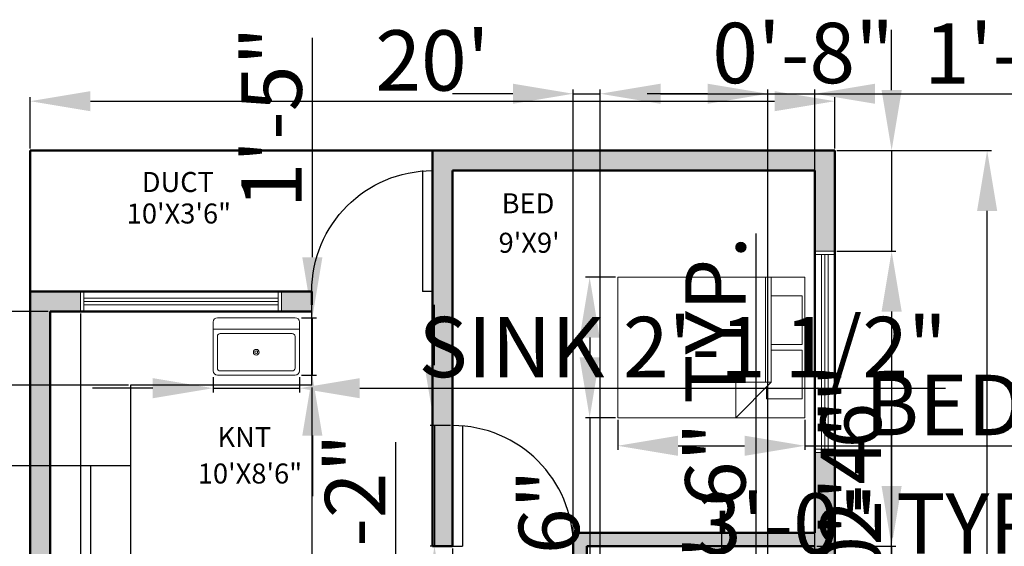
# Model space of a CAD drawing. Units: inches. Extents: x -261 to 409, y 193 to 762.
# Tile 5 of 6: x -35 to 259, y 605 to 762. Entities that reach past the tile are written whole.
import ezdxf

# ---------------------------------------------------------------- set-up
doc = ezdxf.new("R2010")
doc.units = ezdxf.units.IN
for name, color, linetype, lineweight in [('A-ANNO-DIMS', 2, 'Continuous', 18), ('A-AREA-IDEN', 7, 'Continuous', 25), ('A-DOOR', 3, 'Continuous', 25), ('A-FLOR-CASE', 9, 'Continuous', 25), ('A-FLOR-FIXT', 9, 'Continuous', 18), ('A-FURN', 8, 'Continuous', 18), ('A-GLAZ', 4, 'Continuous', 18), ('A-WALL', 7, 'Continuous', 50), ('A-WALL-PATT', 8, 'Continuous', 13)]:
    doc.layers.add(name, color=color, linetype=linetype, lineweight=lineweight)
doc.styles.get("Standard").update_dxf_attribs({"font": 'arial.ttf'})
doc.dimstyles.new('ISO-25', dxfattribs={"dimtxt": 18, "dimasz": 18, "dimexe": 1.25, "dimexo": 0.625, "dimtad": 1, "dimdec": 1, "dimlunit": 3, "dimtxsty": 'Standard', "dimcen": 2.5, "dimadec": 0, "dimazin": 0, "dimtfac": 1, "dimtdec": 1, "dimtmove": 0, "dimatfit": 3, "dimfxl": 1, "dimarcsym": 0})

# ---------------------------------------------------------------- blocks, each defined once
blk = doc.blocks.new('Bed - Queen')
for p, q in [((0, -80.00003), (0, 0)), ((0, 0), (59.99999, 0)), ((59.99999, 0), (59.99999, -80.00003)), ((7.99999, -1.2), (28.79998, -1.2)), ((7.99999, -14.4), (7.99999, -1.2)), ((28.79998, -1.2), (28.79998, -14.4)), ((31.19999, -1.2), (51.99999, -1.2)), ((31.19999, -14.4), (31.19999, -1.2)), ((51.99999, -1.2), (51.99999, -16.4)), ((0, -14.4), (44.8, -14.4)), ((44.8, -16.8), (0, -16.8)), ((59.99999, -29.6), (44.8, -14.4)), ((44.8, -14.4), (44.8, -29.6)), ((51.99999, -16.4), (46.79936, -16.4)), ((44.8, -29.6), (59.99999, -29.6)), ((59.99999, -80.00003), (0, -80.00003))]:
    blk.add_line(p, q)
blk = doc.blocks.new('Sink-single - 30 in top')
blk.add_line((-15, -3.999996), (15, -3.999996))
for points in [[(-13.5, 0), (13.5, 0)], [(-15, -18.499996), (-15, -1.5)], [(15, -1.5), (15, -18.499996)], [(-13.5, -17.499996), (-13.5, -6.499996)], [(-12.5, -5.499996), (12.5, -5.499996)], [(13.5, -6.499996), (13.5, -17.499996)], [(13.5, -19.999996), (-13.5, -19.999996)], [(12.5, -18.499996), (-12.5, -18.499996)]]:
    blk.add_lwpolyline(points)
for radius in [1, 0.5]:
    blk.add_circle((0, -11.999996), radius)
for centre, radius, start, end in [((-13.5, -1.5), 1.5, 90, 180), ((13.5, -1.5), 1.5, 0, 90), ((-12.5, -6.499996), 1, 90, 180), ((12.5, -6.499996), 1, 0, 90), ((-13.5, -18.499996), 1.5, 180, 270), ((-12.5, -17.499996), 1, 180, 270), ((12.5, -17.499996), 1, 270, 0), ((13.5, -18.499996), 1.5, 270, 0)]:
    blk.add_arc(centre, radius, start, end)
blk = doc.blocks.new('*D5')
at = {"layer": 'A-ANNO-DIMS', "color": 0, "lineweight": -2, "transparency": 16777216}
for p, q in [((-31.7, 723.89), (-31.7, 739.21)), ((-13.7, 737.96), (190.3, 737.96)), ((208.3, 723.89), (208.3, 739.21))]:
    blk.add_line(p, q, dxfattribs=at)
at = {"layer": 'A-ANNO-DIMS', "color": 0, "transparency": 16777216}
for points in [[(-13.7, 740.96), (-13.7, 734.96), (-31.7, 737.96)], [(190.3, 740.96), (190.3, 734.96), (208.3, 737.96)]]:
    blk.add_solid(points, dxfattribs=at)
at = {"layer": 'Defpoints', "color": 0, "transparency": 16777216}
for p in [(208.3, 737.96), (-31.7, 723.26), (208.3, 723.26)]:
    blk.add_point(p, dxfattribs=at)
at = {"layer": 'A-ANNO-DIMS', "color": 0, "transparency": 16777216, "insert": (88.3, 747.77), "char_height": 18, "attachment_point": 5}
blk.add_mtext("20'", dxfattribs=at)
blk = doc.blocks.new('*D6')
at = {"layer": 'A-ANNO-DIMS', "color": 0, "lineweight": -2, "transparency": 16777216}
for p, q in [((208.93, 723.26), (254.96, 723.26)), ((253.71, 441.26), (253.71, 705.26)), ((208.93, 423.26), (254.96, 423.26))]:
    blk.add_line(p, q, dxfattribs=at)
at = {"layer": 'A-ANNO-DIMS', "color": 0, "transparency": 16777216}
for points in [[(250.71, 705.26), (256.71, 705.26), (253.71, 723.26)], [(250.71, 441.26), (256.71, 441.26), (253.71, 423.26)]]:
    blk.add_solid(points, dxfattribs=at)
at = {"layer": 'Defpoints', "color": 0, "transparency": 16777216}
for p in [(208.3, 723.26), (253.71, 723.26), (208.3, 423.26)]:
    blk.add_point(p, dxfattribs=at)
at = {"layer": 'A-ANNO-DIMS', "color": 0, "transparency": 16777216, "insert": (243.89, 573.26), "char_height": 18, "attachment_point": 5, "rotation": 90}
blk.add_mtext("25'", dxfattribs=at)
blk = doc.blocks.new('DOOR-SWING-36IN')
for p, q in [((0, 3), (36, 3)), ((36, 0), (36, 3)), ((0, 0), (36, 0))]:
    blk.add_line(p, q)
blk.add_arc((36, 0), 36, 90, 180)
blk = doc.blocks.new('WIN-60IN')
for p, q in [((60, 6), (0, 6)), ((0, 6), (0, 0)), ((1, 6), (1, 0)), ((59, 0), (59, 6)), ((60, 0), (60, 6)), ((59, 4), (1, 4)), ((59, 3), (1, 3)), ((0, 0), (60, 0)), ((59, 2), (1, 2))]:
    blk.add_line(p, q)
blk = doc.blocks.new('*D11')
at = {"layer": 'A-ANNO-DIMS', "color": 0, "lineweight": -2, "transparency": 16777216}
for p, q in [((88.9, 659.26), (88.9, 677.26)), ((93.68, 641.26), (87.65, 641.26)), ((88.9, 641.26), (88.9, 605.26)), ((93.68, 605.26), (87.65, 605.26)), ((88.9, 587.26), (88.9, 376.77))]:
    blk.add_line(p, q, dxfattribs=at)
at = {"layer": 'A-ANNO-DIMS', "color": 0, "transparency": 16777216}
for points in [[(85.9, 659.26), (91.9, 659.26), (88.9, 641.26)], [(85.9, 587.26), (91.9, 587.26), (88.9, 605.26)]]:
    blk.add_solid(points, dxfattribs=at)
at = {"layer": 'Defpoints', "color": 0, "transparency": 16777216}
for p in [(94.3, 641.26), (88.9, 605.26), (94.3, 605.26)]:
    blk.add_point(p, dxfattribs=at)
at = {"layer": 'A-ANNO-DIMS', "color": 0, "transparency": 16777216, "insert": (78.96, 473.02), "char_height": 18, "attachment_point": 5, "rotation": 90}
blk.add_mtext('DOOR 3\'-0" TYP.', dxfattribs=at)
blk = doc.blocks.new('*D12')
at = {"layer": 'A-ANNO-DIMS', "color": 0, "lineweight": -2, "transparency": 16777216}
for p, q in [((94.3, 604.64), (94.3, 598.61)), ((130.3, 604.64), (130.3, 598.61)), ((76.3, 599.86), (58.3, 599.86)), ((94.3, 599.86), (130.3, 599.86)), ((148.3, 599.86), (277.26, 599.86))]:
    blk.add_line(p, q, dxfattribs=at)
at = {"layer": 'A-ANNO-DIMS', "color": 0, "transparency": 16777216}
for points in [[(76.3, 602.86), (76.3, 596.86), (94.3, 599.86)], [(148.3, 602.86), (148.3, 596.86), (130.3, 599.86)]]:
    blk.add_solid(points, dxfattribs=at)
at = {"layer": 'Defpoints', "color": 0, "transparency": 16777216}
for p in [(94.3, 605.26), (130.3, 605.26), (130.3, 599.86)]:
    blk.add_point(p, dxfattribs=at)
at = {"layer": 'A-ANNO-DIMS', "color": 0, "transparency": 16777216, "insert": (221.78, 609.69), "char_height": 18, "attachment_point": 5}
blk.add_mtext('3\'-0" TYP.', dxfattribs=at)
blk = doc.blocks.new('*D14')
at = {"layer": 'A-ANNO-DIMS', "color": 0, "lineweight": -2, "transparency": 16777216}
for p, q in [((184.8, 569.26), (184.8, 698.54)), ((180.93, 551.26), (186.05, 551.26)), ((184.8, 521.26), (184.8, 551.26)), ((180.93, 521.26), (186.05, 521.26)), ((184.8, 503.26), (184.8, 485.26))]:
    blk.add_line(p, q, dxfattribs=at)
at = {"layer": 'A-ANNO-DIMS', "color": 0, "transparency": 16777216}
for points in [[(181.8, 569.26), (187.8, 569.26), (184.8, 551.26)], [(181.8, 503.26), (187.8, 503.26), (184.8, 521.26)]]:
    blk.add_solid(points, dxfattribs=at)
at = {"layer": 'Defpoints', "color": 0, "transparency": 16777216}
for p in [(180.3, 551.26), (184.8, 551.26), (180.3, 521.26)]:
    blk.add_point(p, dxfattribs=at)
at = {"layer": 'A-ANNO-DIMS', "color": 0, "transparency": 16777216, "insert": (174.99, 642.9), "char_height": 18, "attachment_point": 5, "rotation": 90}
blk.add_mtext('2\'-6" TYP.', dxfattribs=at)
blk = doc.blocks.new('*D19')
at = {"layer": 'A-ANNO-DIMS', "color": 0, "lineweight": -2, "transparency": 16777216}
for p, q in [((143.56, 642.98), (143.56, 633.98)), ((199.37, 642.98), (199.37, 633.98)), ((161.56, 635.23), (181.37, 635.23)), ((199.37, 635.23), (324.36, 635.23))]:
    blk.add_line(p, q, dxfattribs=at)
at = {"layer": 'A-ANNO-DIMS', "color": 0, "transparency": 16777216}
for points in [[(161.56, 638.23), (161.56, 632.23), (143.56, 635.23)], [(181.37, 638.23), (181.37, 632.23), (199.37, 635.23)]]:
    blk.add_solid(points, dxfattribs=at)
at = {"layer": 'Defpoints', "color": 0, "transparency": 16777216}
for p in [(143.56, 643.61), (199.37, 643.61), (199.37, 635.23)]:
    blk.add_point(p, dxfattribs=at)
at = {"layer": 'A-ANNO-DIMS', "color": 0, "transparency": 16777216, "insert": (270.87, 645.05), "char_height": 18, "attachment_point": 5}
blk.add_mtext('BED 4\'-8"', dxfattribs=at)
blk = doc.blocks.new('*D20')
at = {"layer": 'A-ANNO-DIMS', "color": 0, "lineweight": -2, "transparency": 16777216}
for p, q in [((142.93, 685.47), (133.93, 685.47)), ((135.18, 667.47), (135.18, 661.61)), ((142.93, 643.61), (133.93, 643.61)), ((135.18, 643.61), (135.18, 576.52))]:
    blk.add_line(p, q, dxfattribs=at)
at = {"layer": 'A-ANNO-DIMS', "color": 0, "transparency": 16777216}
for points in [[(132.18, 667.47), (138.18, 667.47), (135.18, 685.47)], [(132.18, 661.61), (138.18, 661.61), (135.18, 643.61)]]:
    blk.add_solid(points, dxfattribs=at)
at = {"layer": 'Defpoints', "color": 0, "transparency": 16777216}
for p in [(143.56, 685.47), (135.18, 643.61), (143.56, 643.61)]:
    blk.add_point(p, dxfattribs=at)
at = {"layer": 'A-ANNO-DIMS', "color": 0, "transparency": 16777216, "insert": (125.36, 601.06), "char_height": 18, "attachment_point": 5, "rotation": 90}
blk.add_mtext('3\'-6"', dxfattribs=at)
blk = doc.blocks.new('*D23')
at = {"layer": 'A-ANNO-DIMS', "color": 0, "lineweight": -2, "transparency": 16777216}
for p, q in [((174.57, 597.13), (174.57, 615.13)), ((176.57, 579.13), (173.32, 579.13)), ((174.57, 579.13), (174.57, 561.62)), ((176.57, 561.62), (173.32, 561.62)), ((174.57, 543.62), (174.57, 384.96))]:
    blk.add_line(p, q, dxfattribs=at)
at = {"layer": 'A-ANNO-DIMS', "color": 0, "transparency": 16777216}
for points in [[(171.57, 597.13), (177.57, 597.13), (174.57, 579.13)], [(171.57, 543.62), (177.57, 543.62), (174.57, 561.62)]]:
    blk.add_solid(points, dxfattribs=at)
at = {"layer": 'Defpoints', "color": 0, "transparency": 16777216}
for p in [(177.2, 579.13), (174.57, 561.62), (177.2, 561.62)]:
    blk.add_point(p, dxfattribs=at)
at = {"layer": 'A-ANNO-DIMS', "color": 0, "transparency": 16777216, "insert": (164.64, 455.29), "char_height": 18, "attachment_point": 5, "rotation": 90}
blk.add_mtext('WC 1\'-5 1/2"', dxfattribs=at)
blk = doc.blocks.new('*D25')
at = {"layer": 'A-ANNO-DIMS', "color": 0, "lineweight": -2, "transparency": 16777216}
for p, q in [((22.88, 655.64), (22.88, 651.15)), ((48.62, 655.64), (48.62, 651.15)), ((4.88, 652.4), (-13.12, 652.4)), ((22.88, 652.4), (48.62, 652.4)), ((66.62, 652.4), (241.26, 652.4))]:
    blk.add_line(p, q, dxfattribs=at)
at = {"layer": 'A-ANNO-DIMS', "color": 0, "transparency": 16777216}
for points in [[(4.88, 655.4), (4.88, 649.4), (22.88, 652.4)], [(66.62, 655.4), (66.62, 649.4), (48.62, 652.4)]]:
    blk.add_solid(points, dxfattribs=at)
at = {"layer": 'Defpoints', "color": 0, "transparency": 16777216}
for p in [(22.88, 656.26), (48.62, 656.26), (48.62, 652.4)]:
    blk.add_point(p, dxfattribs=at)
at = {"layer": 'A-ANNO-DIMS', "color": 0, "transparency": 16777216, "insert": (162.94, 662.33), "char_height": 18, "attachment_point": 5}
blk.add_mtext('SINK 2\'-1 1/2"', dxfattribs=at)
blk = doc.blocks.new('*D26')
at = {"layer": 'A-ANNO-DIMS', "color": 0, "lineweight": -2, "transparency": 16777216}
for p, q in [((52.48, 691.42), (52.48, 756.83)), ((49.25, 673.42), (53.73, 673.42)), ((52.48, 656.26), (52.48, 673.42)), ((49.25, 656.26), (53.73, 656.26)), ((52.48, 638.26), (52.48, 620.26))]:
    blk.add_line(p, q, dxfattribs=at)
at = {"layer": 'A-ANNO-DIMS', "color": 0, "transparency": 16777216}
for points in [[(49.48, 691.42), (55.48, 691.42), (52.48, 673.42)], [(49.48, 638.26), (55.48, 638.26), (52.48, 656.26)]]:
    blk.add_solid(points, dxfattribs=at)
at = {"layer": 'Defpoints', "color": 0, "transparency": 16777216}
for p in [(48.62, 673.42), (52.48, 673.42), (48.62, 656.26)]:
    blk.add_point(p, dxfattribs=at)
at = {"layer": 'A-ANNO-DIMS', "color": 0, "transparency": 16777216, "insert": (42.67, 733.12), "char_height": 18, "attachment_point": 5, "rotation": 90}
blk.add_mtext('1\'-5"', dxfattribs=at)
blk = doc.blocks.new('*D30')
at = {"layer": 'A-ANNO-DIMS', "color": 0, "lineweight": -2, "transparency": 16777216}
for p, q in [((225.22, 741.26), (225.22, 759.26)), ((208.93, 723.26), (226.47, 723.26)), ((225.22, 723.26), (225.22, 693.26)), ((208.93, 693.26), (226.47, 693.26)), ((225.22, 675.26), (225.22, 607.86))]:
    blk.add_line(p, q, dxfattribs=at)
at = {"layer": 'A-ANNO-DIMS', "color": 0, "transparency": 16777216}
for points in [[(222.22, 741.26), (228.22, 741.26), (225.22, 723.26)], [(222.22, 675.26), (228.22, 675.26), (225.22, 693.26)]]:
    blk.add_solid(points, dxfattribs=at)
at = {"layer": 'Defpoints', "color": 0, "transparency": 16777216}
for p in [(208.3, 723.26), (208.3, 693.26), (225.22, 693.26)]:
    blk.add_point(p, dxfattribs=at)
at = {"layer": 'A-ANNO-DIMS', "color": 0, "transparency": 16777216, "insert": (215.4, 632.56), "char_height": 18, "attachment_point": 5, "rotation": 90}
blk.add_mtext('2\'-6"', dxfattribs=at)
blk = doc.blocks.new('*D31')
at = {"layer": 'A-ANNO-DIMS', "color": 0, "lineweight": -2, "transparency": 16777216}
for p, q in [((-25.7, 674.64), (-25.7, 405.1)), ((-16.7, 674.64), (-16.7, 405.1)), ((-43.7, 406.35), (-61.7, 406.35)), ((-25.7, 406.35), (-16.7, 406.35)), ((1.3, 406.35), (68.4, 406.35))]:
    blk.add_line(p, q, dxfattribs=at)
at = {"layer": 'A-ANNO-DIMS', "color": 0, "transparency": 16777216}
for points in [[(-43.7, 409.35), (-43.7, 403.35), (-25.7, 406.35)], [(1.3, 409.35), (1.3, 403.35), (-16.7, 406.35)]]:
    blk.add_solid(points, dxfattribs=at)
at = {"layer": 'Defpoints', "color": 0, "transparency": 16777216}
for p in [(-25.7, 675.26), (-16.7, 675.26), (-16.7, 406.35)]:
    blk.add_point(p, dxfattribs=at)
at = {"layer": 'A-ANNO-DIMS', "color": 0, "transparency": 16777216, "insert": (43.85, 416.17), "char_height": 18, "attachment_point": 5}
blk.add_mtext('0\'-9"', dxfattribs=at)
blk = doc.blocks.new('*D33')
at = {"layer": 'A-ANNO-DIMS', "color": 0, "lineweight": -2, "transparency": 16777216}
for p, q in [((225.22, 623.26), (225.22, 641.26)), ((202.93, 605.26), (226.47, 605.26)), ((225.22, 605.26), (225.22, 589.26)), ((202.93, 589.26), (226.47, 589.26)), ((225.22, 571.26), (225.22, 505.86))]:
    blk.add_line(p, q, dxfattribs=at)
at = {"layer": 'A-ANNO-DIMS', "color": 0, "transparency": 16777216}
for points in [[(222.22, 623.26), (228.22, 623.26), (225.22, 605.26)], [(222.22, 571.26), (228.22, 571.26), (225.22, 589.26)]]:
    blk.add_solid(points, dxfattribs=at)
at = {"layer": 'Defpoints', "color": 0, "transparency": 16777216}
for p in [(202.3, 605.26), (202.3, 589.26), (225.22, 589.26)]:
    blk.add_point(p, dxfattribs=at)
at = {"layer": 'A-ANNO-DIMS', "color": 0, "transparency": 16777216, "insert": (215.55, 529.56), "char_height": 18, "attachment_point": 5, "rotation": 90}
blk.add_mtext('1\'-4"', dxfattribs=at)
blk = doc.blocks.new('*D35')
at = {"layer": 'A-ANNO-DIMS', "color": 0, "lineweight": -2, "transparency": 16777216}
for p, q in [((-48.61, 671.26), (-48.61, 689.26)), ((-2.32, 653.26), (-49.86, 653.26)), ((-48.61, 653.26), (-48.61, 629.26)), ((-2.32, 629.26), (-49.86, 629.26)), ((-48.61, 611.26), (-48.61, 543.86))]:
    blk.add_line(p, q, dxfattribs=at)
at = {"layer": 'A-ANNO-DIMS', "color": 0, "transparency": 16777216}
for points in [[(-51.61, 671.26), (-45.61, 671.26), (-48.61, 653.26)], [(-51.61, 611.26), (-45.61, 611.26), (-48.61, 629.26)]]:
    blk.add_solid(points, dxfattribs=at)
at = {"layer": 'Defpoints', "color": 0, "transparency": 16777216}
for p in [(-1.7, 653.26), (-48.61, 629.26), (-1.7, 629.26)]:
    blk.add_point(p, dxfattribs=at)
at = {"layer": 'A-ANNO-DIMS', "color": 0, "transparency": 16777216, "insert": (-58.42, 568.56), "char_height": 18, "attachment_point": 5, "rotation": 90}
blk.add_mtext('2\'-0"', dxfattribs=at)
blk = doc.blocks.new('*D36')
at = {"layer": 'A-ANNO-DIMS', "color": 0, "lineweight": -2, "transparency": 16777216}
for p, q in [((-25.7, 628.64), (-25.7, 405.1)), ((-1.7, 628.64), (-1.7, 405.1)), ((-43.7, 406.35), (-61.7, 406.35)), ((-25.7, 406.35), (-1.7, 406.35)), ((16.3, 406.35), (83.71, 406.35))]:
    blk.add_line(p, q, dxfattribs=at)
at = {"layer": 'A-ANNO-DIMS', "color": 0, "transparency": 16777216}
for points in [[(-43.7, 409.35), (-43.7, 403.35), (-25.7, 406.35)], [(16.3, 409.35), (16.3, 403.35), (-1.7, 406.35)]]:
    blk.add_solid(points, dxfattribs=at)
at = {"layer": 'Defpoints', "color": 0, "transparency": 16777216}
for p in [(-25.7, 629.26), (-1.7, 629.26), (-1.7, 406.35)]:
    blk.add_point(p, dxfattribs=at)
at = {"layer": 'A-ANNO-DIMS', "color": 0, "transparency": 16777216, "insert": (59.01, 416.17), "char_height": 18, "attachment_point": 5}
blk.add_mtext('2\'-0"', dxfattribs=at)
blk = doc.blocks.new('*D38')
at = {"layer": 'A-ANNO-DIMS', "color": 0, "lineweight": -2, "transparency": 16777216}
for p, q in [((225.22, 579.26), (225.22, 646.36)), ((202.93, 561.26), (226.47, 561.26)), ((225.22, 557.26), (225.22, 561.26)), ((202.93, 557.26), (226.47, 557.26)), ((225.22, 539.26), (225.22, 521.26))]:
    blk.add_line(p, q, dxfattribs=at)
at = {"layer": 'A-ANNO-DIMS', "color": 0, "transparency": 16777216}
for points in [[(222.22, 579.26), (228.22, 579.26), (225.22, 561.26)], [(222.22, 539.26), (228.22, 539.26), (225.22, 557.26)]]:
    blk.add_solid(points, dxfattribs=at)
at = {"layer": 'Defpoints', "color": 0, "transparency": 16777216}
for p in [(202.3, 561.26), (225.22, 561.26), (202.3, 557.26)]:
    blk.add_point(p, dxfattribs=at)
at = {"layer": 'A-ANNO-DIMS', "color": 0, "transparency": 16777216, "insert": (215.4, 621.81), "char_height": 18, "attachment_point": 5, "rotation": 90}
blk.add_mtext('0\'-4"', dxfattribs=at)
blk = doc.blocks.new('*D42')
at = {"layer": 'A-ANNO-DIMS', "color": 0, "lineweight": -2, "transparency": 16777216}
for p, q in [((112.3, 740.18), (94.3, 740.18)), ((130.3, 461.89), (130.3, 741.43)), ((130.3, 740.18), (138.3, 740.18)), ((138.3, 461.89), (138.3, 741.43)), ((156.3, 740.18), (223.4, 740.18))]:
    blk.add_line(p, q, dxfattribs=at)
at = {"layer": 'A-ANNO-DIMS', "color": 0, "transparency": 16777216}
for points in [[(112.3, 743.18), (112.3, 737.18), (130.3, 740.18)], [(156.3, 743.18), (156.3, 737.18), (138.3, 740.18)]]:
    blk.add_solid(points, dxfattribs=at)
at = {"layer": 'Defpoints', "color": 0, "transparency": 16777216}
for p in [(138.3, 740.18), (130.3, 461.26), (138.3, 461.26)]:
    blk.add_point(p, dxfattribs=at)
at = {"layer": 'A-ANNO-DIMS', "color": 0, "transparency": 16777216, "insert": (198.85, 749.99), "char_height": 18, "attachment_point": 5}
blk.add_mtext('0\'-8"', dxfattribs=at)
blk = doc.blocks.new('*D43')
at = {"layer": 'A-ANNO-DIMS', "color": 0, "lineweight": -2, "transparency": 16777216}
for p, q in [((77.39, 569.26), (77.39, 636.35)), ((93.68, 569.26), (76.14, 569.26)), ((77.39, 549.26), (77.39, 551.26)), ((93.68, 531.26), (76.14, 531.26))]:
    blk.add_line(p, q, dxfattribs=at)
at = {"layer": 'A-ANNO-DIMS', "color": 0, "transparency": 16777216}
for points in [[(74.39, 551.26), (80.39, 551.26), (77.39, 569.26)], [(74.39, 549.26), (80.39, 549.26), (77.39, 531.26)]]:
    blk.add_solid(points, dxfattribs=at)
at = {"layer": 'Defpoints', "color": 0, "transparency": 16777216}
for p in [(77.39, 569.26), (94.3, 569.26), (94.3, 531.26)]:
    blk.add_point(p, dxfattribs=at)
at = {"layer": 'A-ANNO-DIMS', "color": 0, "transparency": 16777216, "insert": (67.57, 611.81), "char_height": 18, "attachment_point": 5, "rotation": 90}
blk.add_mtext('3\'-2"', dxfattribs=at)
blk = doc.blocks.new('*D44')
at = {"layer": 'A-ANNO-DIMS', "color": 0, "lineweight": -2, "transparency": 16777216}
for p, q in [((170.32, 740.18), (152.32, 740.18)), ((188.32, 562.25), (188.32, 741.43)), ((188.32, 740.18), (202.3, 740.18)), ((202.3, 561.89), (202.3, 741.43)), ((220.3, 740.18), (285.71, 740.18))]:
    blk.add_line(p, q, dxfattribs=at)
at = {"layer": 'A-ANNO-DIMS', "color": 0, "transparency": 16777216}
for points in [[(170.32, 743.18), (170.32, 737.18), (188.32, 740.18)], [(220.3, 743.18), (220.3, 737.18), (202.3, 740.18)]]:
    blk.add_solid(points, dxfattribs=at)
at = {"layer": 'Defpoints', "color": 0, "transparency": 16777216}
for p in [(202.3, 740.18), (188.32, 561.62), (202.3, 561.26)]:
    blk.add_point(p, dxfattribs=at)
at = {"layer": 'A-ANNO-DIMS', "color": 0, "transparency": 16777216, "insert": (262.01, 749.84), "char_height": 18, "attachment_point": 5}
blk.add_mtext('1\'-2"', dxfattribs=at)
blk = doc.blocks.new('*D45')
at = {"layer": 'A-ANNO-DIMS', "color": 0, "lineweight": -2, "transparency": 16777216}
for p, q in [((-48.61, 693.26), (-48.61, 711.26)), ((-26.32, 675.26), (-49.86, 675.26)), ((-48.61, 675.26), (-48.61, 653.26)), ((-2.32, 653.26), (-49.86, 653.26)), ((-48.61, 635.26), (-48.61, 555.87))]:
    blk.add_line(p, q, dxfattribs=at)
at = {"layer": 'A-ANNO-DIMS', "color": 0, "transparency": 16777216}
for points in [[(-51.61, 693.26), (-45.61, 693.26), (-48.61, 675.26)], [(-51.61, 635.26), (-45.61, 635.26), (-48.61, 653.26)]]:
    blk.add_solid(points, dxfattribs=at)
at = {"layer": 'Defpoints', "color": 0, "transparency": 16777216}
for p in [(-25.7, 675.26), (-48.61, 653.26), (-1.7, 653.26)]:
    blk.add_point(p, dxfattribs=at)
at = {"layer": 'A-ANNO-DIMS', "color": 0, "transparency": 16777216, "insert": (-58.42, 586.57), "char_height": 18, "attachment_point": 5, "rotation": 90}
blk.add_mtext('1\'-10"', dxfattribs=at)
blk = doc.blocks.new('*D46')
at = {"layer": 'A-ANNO-DIMS', "color": 0, "lineweight": -2, "transparency": 16777216}
for p, q in [((-1.7, 652.64), (-1.7, 405.1)), ((52.3, 652.64), (52.3, 405.1)), ((16.3, 406.35), (34.3, 406.35))]:
    blk.add_line(p, q, dxfattribs=at)
at = {"layer": 'A-ANNO-DIMS', "color": 0, "transparency": 16777216}
for points in [[(16.3, 409.35), (16.3, 403.35), (-1.7, 406.35)], [(34.3, 409.35), (34.3, 403.35), (52.3, 406.35)]]:
    blk.add_solid(points, dxfattribs=at)
at = {"layer": 'Defpoints', "color": 0, "transparency": 16777216}
for p in [(-1.7, 653.26), (52.3, 653.26), (52.3, 406.35)]:
    blk.add_point(p, dxfattribs=at)
at = {"layer": 'A-ANNO-DIMS', "color": 0, "transparency": 16777216, "insert": (25.3, 416.17), "char_height": 18, "attachment_point": 5}
blk.add_mtext('4\'-6"', dxfattribs=at)

msp = doc.modelspace()

# ---------------------------------------------------------------- hatches: boundary and pattern name
at = {"layer": 'A-WALL-PATT'}
h = msp.add_hatch(color=256, dxfattribs=at)
h.dxf.hatch_style = 1
h.paths.add_polyline_path([(-25.7, 675.26), (-16.7, 675.26), (-16.7, 681.26), (-31.7, 681.26), (-31.7, 423.26), (-14.2, 423.26), (-14.2, 429.26), (-25.7, 429.26), (-25.7, 569.26), (52.3, 569.26), (88.3, 569.26), (94.3, 569.26), (94.3, 573.26), (52.3, 573.26), (-25.7, 573.26), (-25.7, 575.26)])
h.paths.add_polyline_path([(94.3, 429.26), (58.3, 429.26), (45.8, 429.26), (45.8, 423.26), (94.3, 423.26)])
h.paths.add_polyline_path([(208.3, 533.26), (202.3, 533.26), (202.3, 521.26), (150.3, 521.26), (94.3, 521.26), (94.3, 531.26), (88.3, 531.26), (88.3, 465.26), (94.3, 465.26), (94.3, 517.26), (150.3, 517.26), (202.3, 517.26), (202.3, 429.26), (130.3, 429.26), (130.3, 423.26), (208.3, 423.26)])
h.paths.add_polyline_path([(208.3, 577.26), (202.3, 577.26), (202.3, 561.26), (130.3, 561.26), (130.3, 557.26), (150.3, 557.26), (150.3, 551.26), (154.3, 551.26), (154.3, 557.26), (202.3, 557.26), (202.3, 545.26), (208.3, 545.26)])
h.paths.add_polyline_path([(208.3, 633.26), (202.3, 633.26), (202.3, 609.26), (130.3, 609.26), (130.3, 605.26), (130.3, 591.26), (134.3, 591.26), (134.3, 605.26), (202.3, 605.26), (202.3, 589.26), (208.3, 589.26)])
h.paths.add_polyline_path([(208.3, 723.26), (88.3, 723.26), (88.3, 605.26), (94.3, 605.26), (94.3, 641.26), (94.3, 717.26), (202.3, 717.26), (202.3, 693.26), (208.3, 693.26)])
h.paths.add_polyline_path([(52.3, 681.26), (43.3, 681.26), (43.3, 675.26), (52.3, 675.26), (52.3, 677.26)], flags=17)

# ---------------------------------------------------------------- linework, layer by layer
at = {"layer": 'A-FLOR-CASE'}
for p, q in [((52.3, 653.26), (52.3, 677.26)), ((-1.7, 653.26), (-1.7, 629.26)), ((52.3, 653.26), (-1.7, 653.26)), ((-1.7, 629.26), (-25.7, 629.26)), ((-13.7, 629.26), (-13.7, 579.26))]:
    msp.add_line(p, q, dxfattribs=at)
at = {"layer": 'A-WALL'}
for p, q in [((208.3, 723.26), (-31.7, 723.26)), ((-31.7, 723.26), (-31.7, 423.26)), ((88.3, 723.26), (88.3, 605.26)), ((208.3, 423.26), (208.3, 723.26)), ((94.3, 717.26), (94.3, 605.26)), ((202.3, 717.26), (94.3, 717.26)), ((202.3, 609.26), (202.3, 717.26)), ((52.3, 681.26), (-31.7, 681.26)), ((52.3, 681.26), (52.3, 677.26)), ((-25.7, 675.26), (-25.7, 575.26)), ((52.3, 675.26), (-25.7, 675.26)), ((202.3, 609.26), (130.3, 609.26)), ((130.3, 609.26), (130.3, 605.26)), ((94.3, 605.26), (88.3, 605.26)), ((130.3, 591.26), (130.3, 605.26)), ((202.3, 605.26), (134.3, 605.26)), ((134.3, 591.26), (134.3, 605.26))]:
    msp.add_line(p, q, dxfattribs=at)

# ---------------------------------------------------------------- block references
at = {"layer": 'A-DOOR', "extrusion": (0, 0, -1), "zscale": -1, "rotation": 270}
msp.add_blockref('DOOR-SWING-36IN', (-88.3, 717.26), dxfattribs=at)
at = {"layer": 'A-DOOR', "rotation": 270}
msp.add_blockref('DOOR-SWING-36IN', (94.3, 641.26), dxfattribs=at)
at = {"layer": 'A-FLOR-FIXT', "xscale": 0.8579498762486251, "yscale": 0.8579498762486251, "zscale": 0.8579498762486251}
msp.add_blockref('Sink-single - 30 in top', (35.75, 673.42), dxfattribs=at)
at = {"layer": 'A-FURN', "xscale": 0.6976867227961034, "yscale": 0.6976867227961034, "zscale": 0.6976867227961034, "rotation": 270}
msp.add_blockref('Bed - Queen', (199.37, 685.47), dxfattribs=at)
at = {"layer": 'A-GLAZ'}
for p, rotation in [((202.3, 693.26), 270.0000000000004), ((43.3, 681.26), 180)]:
    msp.add_blockref('WIN-60IN', p, dxfattribs=dict(at, rotation=rotation))

# ---------------------------------------------------------------- texts
at = {"layer": 'A-AREA-IDEN', "char_height": 5.965, "attachment_point": 1}
for s, insert in [('DUCT', (1.61, 716.85)), ('10\'X3\'6"', (-2.87, 707.46)), ('BED', (108.92, 710.5)), ("9'X9'", (108.01, 698.74)), ('KNT', (24.2, 640.81)), ('10\'X8\'6"', (18.32, 629.95))]:
    msp.add_mtext_dynamic_manual_height_columns(s, width=143.7583, gutter_width=29.83, heights=[0], dxfattribs=dict(at, insert=insert))

# ---------------------------------------------------------------- dimensions: what is measured, and where the dimension line sits
at = {"layer": 'A-ANNO-DIMS'}
for base, p1, p2, override, picture, middle in [((138.3, 740.18), (130.3, 461.26), (138.3, 461.26), {"dimdec": 1, "dimlfac": 1, "dimrnd": 0, "dimzin": 1, "dimdsep": 46, "dimlunit": 4, "dimfrac": 2}, '*D42', (198.85, 749.99)), ((202.3, 740.18), (188.32, 561.62), (202.3, 561.26), {"dimdec": 1, "dimlfac": 1, "dimrnd": 0, "dimzin": 1, "dimdsep": 46, "dimlunit": 4, "dimfrac": 2}, '*D44', (262.01, 749.84)), ((208.3, 737.96), (-31.7, 723.26), (208.3, 723.26), {"dimclrd": 0, "dimclre": 0, "dimclrt": 0}, '*D5', (88.3, 747.77)), ((-16.7, 406.35), (-25.7, 675.26), (-16.7, 675.26), {"dimdec": 1, "dimlfac": 1, "dimrnd": 0, "dimzin": 1, "dimdsep": 46, "dimlunit": 4, "dimfrac": 2}, '*D31', (43.85, 416.17)), ((52.3, 406.35), (-1.7, 653.26), (52.3, 653.26), {"dimdec": 1, "dimlfac": 1, "dimrnd": 0, "dimzin": 1, "dimdsep": 46, "dimlunit": 4, "dimfrac": 2}, '*D46', (25.3, 416.17)), ((-1.7, 406.35), (-25.7, 629.26), (-1.7, 629.26), {"dimdec": 1, "dimlfac": 1, "dimrnd": 0, "dimzin": 1, "dimdsep": 46, "dimlunit": 4, "dimfrac": 2}, '*D36', (59.01, 416.17))]:
    dim = msp.add_linear_dim(base=base, p1=p1, p2=p2, dimstyle='ISO-25', override=override, dxfattribs=at)
    dim.commit()
    dim.dimension.update_dxf_attribs({"geometry": picture, "text_midpoint": middle})
for base, p1, p2, angle, override, picture, middle in [((52.48, 673.42), (48.62, 656.26), (48.62, 673.42), 90, {"dimdec": 1, "dimlfac": 1, "dimrnd": 0, "dimzin": 1, "dimdsep": 46, "dimlunit": 4, "dimfrac": 2}, '*D26', (42.67, 733.12)), ((225.22, 693.26), (208.3, 723.26), (208.3, 693.26), 90, {"dimdec": 1, "dimlfac": 1, "dimrnd": 0, "dimzin": 1, "dimdsep": 46, "dimlunit": 4, "dimfrac": 2}, '*D30', (215.4, 632.56)), ((253.71, 723.26), (208.3, 423.26), (208.3, 723.26), 90, {"dimclrd": 0, "dimclre": 0, "dimclrt": 0}, '*D6', (243.89, 573.26)), ((-48.61, 653.26), (-25.7, 675.26), (-1.7, 653.26), 90, {"dimdec": 1, "dimlfac": 1, "dimrnd": 0, "dimzin": 1, "dimdsep": 46, "dimlunit": 4, "dimfrac": 2}, '*D45', (-58.42, 586.57)), ((-48.61, 629.26), (-1.7, 653.26), (-1.7, 629.26), 90, {"dimdec": 1, "dimlfac": 1, "dimrnd": 0, "dimzin": 1, "dimdsep": 46, "dimlunit": 4, "dimfrac": 2}, '*D35', (-58.42, 568.56)), ((135.18, 643.61), (143.56, 685.47), (143.56, 643.61), 270, {"dimdec": 1, "dimlfac": 1, "dimrnd": 0, "dimzin": 1, "dimdsep": 46, "dimlunit": 4, "dimfrac": 2}, '*D20', (125.36, 601.06)), ((225.22, 561.26), (202.3, 557.26), (202.3, 561.26), 90, {"dimdec": 1, "dimlfac": 1, "dimrnd": 0, "dimzin": 1, "dimdsep": 46, "dimlunit": 4, "dimfrac": 2}, '*D38', (215.4, 621.81)), ((225.22, 589.26), (202.3, 605.26), (202.3, 589.26), 90, {"dimdec": 1, "dimlfac": 1, "dimrnd": 0, "dimzin": 1, "dimdsep": 46, "dimlunit": 4, "dimfrac": 2}, '*D33', (215.55, 529.56)), ((77.39, 569.26), (94.3, 531.26), (94.3, 569.26), 90, {"dimdec": 1, "dimlfac": 1, "dimrnd": 0, "dimzin": 1, "dimdsep": 46, "dimlunit": 4, "dimfrac": 2}, '*D43', (67.57, 611.81))]:
    dim = msp.add_linear_dim(base=base, p1=p1, p2=p2, angle=angle, dimstyle='ISO-25', override=override, dxfattribs=at)
    dim.commit()
    dim.dimension.update_dxf_attribs({"geometry": picture, "text_midpoint": middle})
for base, p1, p2, text, picture, middle in [((48.62, 652.4), (22.88, 656.26), (48.62, 656.26), 'SINK <>', '*D25', (162.94, 662.33)), ((199.37, 635.23), (143.56, 643.61), (199.37, 643.61), 'BED <>', '*D19', (270.87, 645.05)), ((130.3, 599.86), (94.3, 605.26), (130.3, 605.26), '<> TYP.', '*D12', (221.78, 609.69))]:
    dim = msp.add_linear_dim(base=base, p1=p1, p2=p2, text=text, dimstyle='ISO-25', override={"dimdec": 1, "dimlfac": 1, "dimrnd": 0, "dimzin": 1, "dimdsep": 46, "dimlunit": 4, "dimfrac": 2}, dxfattribs=at)
    dim.commit()
    dim.dimension.update_dxf_attribs({"geometry": picture, "text_midpoint": middle})
for base, p1, p2, angle, text, picture, middle in [((184.8, 551.26), (180.3, 521.26), (180.3, 551.26), 90, '<> TYP.', '*D14', (174.99, 642.9)), ((88.9, 605.26), (94.3, 641.26), (94.3, 605.26), 270, 'DOOR <> TYP.', '*D11', (78.96, 473.02)), ((174.57, 561.62), (177.2, 579.13), (177.2, 561.62), 270, 'WC <>', '*D23', (164.64, 455.29))]:
    dim = msp.add_linear_dim(base=base, p1=p1, p2=p2, angle=angle, text=text, dimstyle='ISO-25', override={"dimdec": 1, "dimlfac": 1, "dimrnd": 0, "dimzin": 1, "dimdsep": 46, "dimlunit": 4, "dimfrac": 2}, dxfattribs=at)
    dim.commit()
    dim.dimension.update_dxf_attribs({"geometry": picture, "text_midpoint": middle})

doc.saveas('drawing.dxf')
